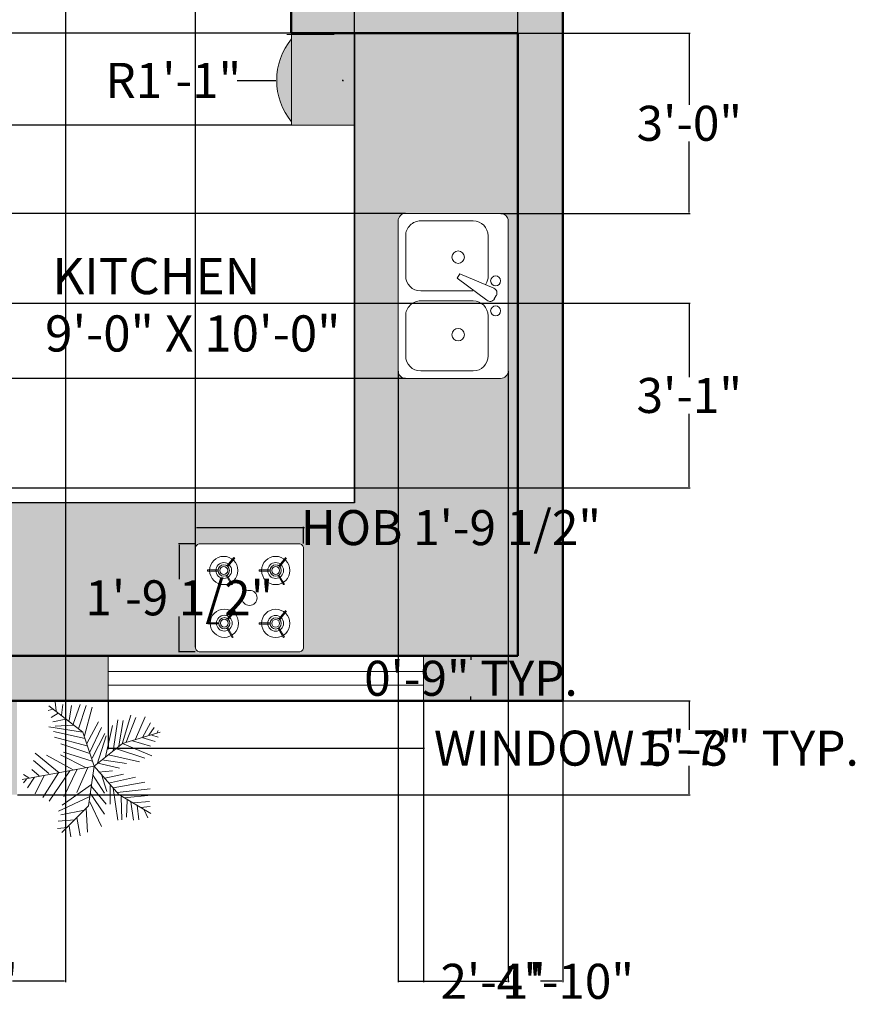
# Model space of a CAD drawing. Units: inches. Extents: x 2974 to 3443, y 2405 to 2963.
# Tile 6 of 13: x 3276 to 3443, y 2411 to 2607. Entities that reach past the tile are written whole.
import ezdxf

# ---------------------------------------------------------------- set-up
doc = ezdxf.new("R2010")
doc.units = ezdxf.units.IN
doc.header["$MEASUREMENT"] = 0
doc.layers.get('0').update_dxf_attribs({"color": 251})
for name, color, linetype, lineweight in [('A-ANNO-DIMS', 2, 'Continuous', 18), ('A-AREA-IDEN', 250, 'Continuous', 25), ('A-EQPM', 32, 'Continuous', 20), ('A-EQPM-PATT', 251, 'Continuous', 13), ('A-FLOR-CASE', 32, 'Continuous', 25), ('A-FLOR-CASE-PATT', 9, 'Continuous', 13), ('A-FLOR-FIXT', 8, 'Continuous', 20), ('A-WALL-PATT', 252, 'Continuous', 13), ('furniture', 32, 'Continuous', 18), ('greenary', 106, 'Continuous', 13), ('walls', 250, 'Continuous', 50), ('windows', 159, 'Continuous', 20)]:
    doc.layers.add(name, color=color, linetype=linetype, lineweight=lineweight)
doc.styles.add('ATT', font='TXT')
doc.styles.get("Standard").update_dxf_attribs({"font": 'arial.ttf'})
doc.dimstyles.get("Standard").update_dxf_attribs({"dimtxt": 7, "dimasz": 0.18, "dimexe": 0.18, "dimexo": 0.0625, "dimgap": 0.09, "dimtad": 0, "dimtih": 1, "dimtoh": 1, "dimzin": 0, "dimdsep": 46, "dimlunit": 3, "dimtxsty": 'Standard', "dimcen": 0.09, "dimadec": 0, "dimazin": 0, "dimtfac": 1, "dimtofl": 0, "dimtmove": 0, "dimatfit": 3, "dimfxl": 1, "dimtolj": 1, "dimtzin": 0, "dimarcsym": 0})

# ---------------------------------------------------------------- blocks, each defined once
blk = doc.blocks.new('15PSNK10')
at = {"color": 0, "linetype": 'ByBlock'}
for p, q in [((20.5, 16.5), (1.5, 16.5)), ((0, 15), (0, -15)), ((7, 15), (17.5, 15)), ((22, -15), (22, 15)), ((4, 4), (4, 12)), ((20.5, 12), (20.5, 4)), ((2.37, -0.1), (2.77, 0.6)), ((10.18, -3.57), (4.27, 0.87)), ((17.5, 1), (7, 1)), ((2.88, -1.54), (9.68, -4.43)), ((7.04, -1), (17.5, -1)), ((9.68, -4.43), (10.18, -3.57)), ((4, -12), (4, -4)), ((20.5, -4), (20.5, -12)), ((17.5, -15), (7, -15)), ((1.5, -16.5), (20.5, -16.5))]:
    blk.add_line(p, q, dxfattribs=at)
for centre, radius in [((10, 7.75), 1.25), ((2.5, 3), 1), ((2.5, -3), 1), ((10, -7.75), 1.25)]:
    blk.add_circle(centre, radius, dxfattribs=at)
for centre, radius, start, end in [((1.5, 15), 1.5, 90, 180), ((20.5, 15), 1.5, 0, 90), ((7, 12), 3, 90, 180), ((17.5, 12), 3, 0, 90), ((7, 4), 3, 180, 270), ((17.5, 4), 3, 270, 0), ((3.63, 0.1), 1, 50.5377, 150), ((3.23, -0.6), 1, 150, 249.4623), ((17.5, -4), 3, 0, 90), ((7, -4), 3, 146.607, 180), ((7, -12), 3, 180, 270), ((17.5, -12), 3, 270, 0), ((1.5, -15), 1.5, 180, 270), ((20.5, -15), 1.5, 270, 0)]:
    blk.add_arc(centre, radius, start, end, dxfattribs=at)
at = {"color": 0, "linetype": 'ByBlock', "style": 'ATT'}
for tag, p, flags in [('ITEM', (0, -26), 3), ('ROOM_NUMBER', (0, -35), 1)]:
    blk.add_attdef(tag, p, '', height=6, dxfattribs=dict(at, flags=flags))
blk = doc.blocks.new('4bstove')
at = {"layer": 'furniture'}
for p, q in [((1452.73, 1446.21), (1452.73, 1448.61)), ((1452.98, 1446.22), (1452.98, 1448.61)), ((1464.44, 1446.34), (1464.44, 1448.73)), ((1464.69, 1446.34), (1464.69, 1448.73)), ((1451.74, 1444.45), (1449.67, 1443.25)), ((1451.87, 1444.23), (1449.79, 1443.04)), ((1453.75, 1444.08), (1455.58, 1442.54)), ((1453.91, 1444.27), (1455.74, 1442.73)), ((1463.45, 1444.58), (1461.38, 1443.38)), ((1463.57, 1444.36), (1461.5, 1443.17)), ((1465.46, 1444.21), (1467.29, 1442.67)), ((1465.62, 1444.4), (1467.45, 1442.86)), ((1452.69, 1434.81), (1452.69, 1437.2)), ((1452.94, 1434.81), (1452.94, 1437.2)), ((1464.44, 1434.81), (1464.44, 1437.2)), ((1464.69, 1434.81), (1464.69, 1437.2)), ((1451.7, 1433.04), (1449.63, 1431.85)), ((1451.82, 1432.83), (1449.75, 1431.63)), ((1453.87, 1432.86), (1455.7, 1431.33)), ((1463.45, 1433.04), (1461.38, 1431.85)), ((1463.57, 1432.83), (1461.5, 1431.63)), ((1465.62, 1432.86), (1467.45, 1431.33)), ((1453.71, 1432.67), (1455.54, 1431.13)), ((1465.46, 1432.67), (1467.29, 1431.13))]:
    blk.add_line(p, q, dxfattribs=at)
for points in [[(1447.5, 1427.38), (1469.5, 1427.38, 0.414214), (1470.5, 1428.38), (1470.5, 1450.38, 0.414214), (1469.5, 1451.38), (1447.5, 1451.38, 0.414214), (1446.5, 1450.38), (1446.5, 1428.38, 0.414214)], [(1465.46, 1445.1, 1), (1463.71, 1445.1, 1)], [(1453.75, 1444.97, 1), (1452, 1444.97, 1)], [(1453.71, 1433.56, 1), (1451.96, 1433.56, 1)], [(1465.46, 1433.56, 1), (1463.71, 1433.56, 1)]]:
    blk.add_lwpolyline(points, format="xyb", close=True, dxfattribs=at)
for points in [[(1454.12, 1444.97, 1), (1451.62, 1444.97, 1), (1454.12, 1444.97, 1)], [(1465.83, 1445.1, 1), (1463.33, 1445.1, 1), (1465.83, 1445.1, 1)], [(1454.08, 1433.56, 1), (1451.58, 1433.56, 1), (1454.08, 1433.56, 1)], [(1465.83, 1433.56, 1), (1463.33, 1433.56, 1), (1465.83, 1433.56, 1)]]:
    blk.add_lwpolyline(points, format="xyb", dxfattribs=at)
for centre, radius in [((1452.87, 1444.97), 3.14), ((1464.58, 1445.1), 3.14), ((1452.87, 1444.97), 1.75), ((1464.58, 1445.1), 1.75), ((1458.5, 1439.38), 1.67), ((1452.83, 1433.56), 3.14), ((1452.83, 1433.56), 1.75), ((1464.58, 1433.56), 3.14), ((1464.58, 1433.56), 1.75)]:
    blk.add_circle(centre, radius, dxfattribs=at)
for centre, start, end in [((1452.87, 1444.97), 88.2645, 92.2039), ((1464.58, 1445.1), 88.2645, 92.2039), ((1452.87, 1444.97), 208.188, 212.1274), ((1452.87, 1444.97), 318.1018, 322.0412), ((1464.58, 1445.1), 208.188, 212.1274), ((1464.58, 1445.1), 318.1018, 322.0412), ((1452.83, 1433.56), 88.2645, 92.2039), ((1464.58, 1433.56), 88.2645, 92.2039)]:
    blk.add_arc(centre, 3.64, start, end, dxfattribs=at)
blk = doc.blocks.new('stove')
at = {"layer": 'furniture', "xscale": 0.9, "yscale": 0.9, "zscale": 0.9, "rotation": 89.99999999999999}
blk.add_blockref('4bstove', (1295.44, -1312.65), dxfattribs=at)
blk = doc.blocks.new('*U13')
for p, q in [((-10.186, 53.64), (-13.084, 55.962)), ((0, 0), (-10.5, 57)), ((-9.099, 51.782), (-6.563, 55.962)), ((-8.737, 47.138), (-17.069, 52.711)), ((-7.65, 43.423), (-2.578, 49.46)), ((-5.839, 35.992), (4.667, 48.067)), ((-5.114, 28.097), (-24.676, 40.636)), ((-7.288, 39.707), (-21.778, 46.673)), ((-5.114, 27.632), (10.463, 46.673)), ((-3.665, 19.273), (-27.574, 35.527)), ((-2.941, 16.486), (8.652, 37.85)), ((16.259, 5.805), (23.142, 31.348)), ((22.055, 7.198), (27.489, 32.277)), ((27, 9), (48, 36)), ((27.127, 9.056), (31.112, 35.992)), ((35.096, 32.741), (37.27, 22.524)), ((38.719, 34.134), (41.979, 28.561)), ((44.153, 36.456), (45.239, 32.741)), ((-31.5, 4.5), (-52.5, 25.5)), ((-48.585, 21.131), (-49.309, 29.026)), ((-43.513, 28.561), (-42.427, 15.558)), ((-38.442, 26.239), (-34.819, 7.663)), ((-35.544, 28.097), (-24.314, 3.947)), ((-14.533, 2.09), (-30.834, 25.31)), ((-24.314, 23.917), (-2.941, 13.7)), ((-1.129, 6.734), (9.014, 26.704)), ((3.942, 1.625), (11.187, 24.381)), ((10.101, 3.483), (17.708, 26.239)), ((31.836, 30.883), (32.561, 16.486)), ((40.53, 25.775), (48.862, 24.846)), ((43.791, 29.954), (51.036, 30.883)), ((-47.498, 19.737), (-55.83, 18.344)), ((33.285, 16.486), (48.862, 10.913)), ((36.183, 19.737), (48.137, 17.88)), ((-40.615, 13.7), (-55.105, 10.913)), ((-20.691, 13.7), (-1.129, 4.876)), ((0, 0), (27, 9)), ((29.662, 12.307), (48.137, 6.269)), ((-33.37, 6.269), (-52.207, 5.34)), ((-28.299, 3.483), (-47.86, -5.805)), ((-21.416, 3.018), (-38.079, -8.128)), ((0, 0), (-31.5, 4.5)), ((-15.982, 2.09), (-30.11, -9.521)), ((0, 0), (-22.5, -19.5)), ((-6.563, 1.161), (-21.416, -8.128)), ((0, 0), (18, -22.5)), ((6.478, 1.625), (26.04, -8.592)), ((11.187, 3.483), (30.749, -5.805)), ((18.07, 5.805), (35.096, -3.483)), ((24.229, 7.663), (46.688, 1.625)), ((-6.563, -5.805), (-19.967, -9.985)), ((-4.752, -3.483), (-3.665, -14.629)), ((2.493, -3.019), (-1.491, -20.202)), ((1.769, -2.555), (24.229, -9.521)), ((5.029, -6.27), (2.131, -25.775)), ((-17.431, -15.094), (-42.789, -18.809)), ((-15.257, -12.772), (-30.11, -12.772)), ((-17.069, -15.094), (-12.721, -40.172)), ((-13.446, -11.378), (-8.737, -32.741)), ((-9.461, -8.592), (-6.201, -23.453)), ((9.014, -11.378), (3.58, -35.992)), ((7.565, -9.056), (32.198, -14.629)), ((12.274, -15.094), (36.907, -18.809)), ((-24.314, -21.596), (-42.427, -22.06)), ((-22.5, -19.5), (-37.5, -45)), ((-20.691, -18.345), (-17.793, -44.352)), ((14.085, -16.951), (6.478, -40.172)), ((18.07, -22.524), (8.289, -45.745)), ((16.259, -19.738), (36.183, -22.989)), ((18, -22.5), (27, -52.5)), ((18.433, -22.524), (40.53, -29.026)), ((-28.299, -29.026), (-42.789, -31.348)), ((-26.849, -26.24), (-40.253, -25.775)), ((-29.023, -30.884), (-27.936, -43.887)), ((-25.038, -23.918), (-22.865, -45.281)), ((20.244, -30.419), (15.897, -44.816)), ((19.157, -25.311), (38.719, -33.206)), ((-30.834, -34.135), (-42.427, -35.528)), ((-32.646, -36.921), (-31.921, -44.352)), ((22.78, -37.85), (19.519, -48.532)), ((21.331, -32.741), (39.081, -40.636)), ((22.78, -38.314), (34.372, -44.816)), ((-34.457, -39.708), (-40.978, -42.494)), ((24.591, -45.745), (23.142, -50.854)), ((24.591, -43.423), (30.749, -47.603)), ((26.764, -49.925), (28.213, -50.854))]:
    blk.add_line(p, q)
blk = doc.blocks.new('WIN-63IN')
for p, q in [((0, 0), (0, -9)), ((63.13, 0), (0, 0)), ((0, 0), (0, -3.12)), ((63.13, -9), (63.13, 0)), ((0, -3.12), (63.13, -3.12)), ((63.13, -3.12), (63.13, -5.89)), ((63.13, -5.89), (0, -5.89)), ((0, -9), (63.13, -9))]:
    blk.add_line(p, q)
blk = doc.blocks.new('*D39')
at = {"layer": 'A-ANNO-DIMS', "color": 0, "lineweight": -2, "transparency": 16777216}
for p, q in [((3293.36, 2471.13), (3293.36, 2461.54)), ((3356.49, 2471.13), (3356.49, 2461.54)), ((3293.54, 2461.72), (3356.31, 2461.72)), ((3356.49, 2461.72), (3356.67, 2461.72))]:
    blk.add_line(p, q, dxfattribs=at)
at = {"layer": 'A-ANNO-DIMS', "color": 0, "transparency": 16777216}
for points in [[(3293.54, 2461.75), (3293.54, 2461.69), (3293.36, 2461.72)], [(3356.31, 2461.75), (3356.31, 2461.69), (3356.49, 2461.72)]]:
    blk.add_solid(points, dxfattribs=at)
at = {"layer": 'Defpoints', "color": 0, "transparency": 16777216}
for p in [(3293.36, 2471.19), (3356.49, 2471.19), (3356.49, 2461.72)]:
    blk.add_point(p, dxfattribs=at)
at = {"layer": 'A-ANNO-DIMS', "color": 0, "transparency": 16777216, "insert": (3401.05, 2461.72), "char_height": 7, "attachment_point": 5}
blk.add_mtext('\\A1;WINDOW 5\'-3" TYP.', dxfattribs=at)
blk = doc.blocks.new('*D40')
at = {"layer": 'A-ANNO-DIMS', "color": 0, "lineweight": -2, "transparency": 16777216}
for p, q in [((3356.55, 2480.19), (3366.14, 2480.19)), ((3365.96, 2480.01), (3365.96, 2479.35)), ((3356.55, 2471.19), (3366.14, 2471.19)), ((3365.96, 2471.37), (3365.96, 2472.02))]:
    blk.add_line(p, q, dxfattribs=at)
at = {"layer": 'A-ANNO-DIMS', "color": 0, "transparency": 16777216}
for points in [[(3365.93, 2480.01), (3365.99, 2480.01), (3365.96, 2480.19)], [(3365.93, 2471.37), (3365.99, 2471.37), (3365.96, 2471.19)]]:
    blk.add_solid(points, dxfattribs=at)
at = {"layer": 'Defpoints', "color": 0, "transparency": 16777216}
for p in [(3356.49, 2480.19), (3365.96, 2480.19), (3356.49, 2471.19)]:
    blk.add_point(p, dxfattribs=at)
at = {"layer": 'A-ANNO-DIMS', "color": 0, "transparency": 16777216, "insert": (3365.96, 2475.69), "char_height": 7, "attachment_point": 5}
blk.add_mtext('\\A1;0\'-9" TYP.', dxfattribs=at)
blk = doc.blocks.new('*D43')
at = {"layer": 'A-ANNO-DIMS', "color": 0, "lineweight": -2, "transparency": 16777216}
for p, q in [((3310.86, 2502.63), (3310.86, 2505.99)), ((3311.04, 2505.81), (3332.28, 2505.81)), ((3332.46, 2502.63), (3332.46, 2505.99)), ((3332.46, 2505.81), (3332.64, 2505.81))]:
    blk.add_line(p, q, dxfattribs=at)
at = {"layer": 'A-ANNO-DIMS', "color": 0, "transparency": 16777216}
for points in [[(3311.04, 2505.84), (3311.04, 2505.78), (3310.86, 2505.81)], [(3332.28, 2505.84), (3332.28, 2505.78), (3332.46, 2505.81)]]:
    blk.add_solid(points, dxfattribs=at)
at = {"layer": 'Defpoints', "color": 0, "transparency": 16777216}
for p in [(3332.46, 2505.81), (3310.86, 2502.57), (3332.46, 2502.57)]:
    blk.add_point(p, dxfattribs=at)
at = {"layer": 'A-ANNO-DIMS', "color": 0, "transparency": 16777216, "insert": (3361.96, 2505.81), "char_height": 7, "attachment_point": 5}
blk.add_mtext('\\A1;HOB 1\'-9 1/2"', dxfattribs=at)
blk = doc.blocks.new('*D44')
at = {"layer": 'A-ANNO-DIMS', "color": 0, "lineweight": -2, "transparency": 16777216}
for p, q in [((3310.8, 2502.57), (3307.44, 2502.57)), ((3307.62, 2502.39), (3307.62, 2495.48)), ((3307.62, 2481.15), (3307.62, 2488.06)), ((3310.8, 2480.97), (3307.44, 2480.97))]:
    blk.add_line(p, q, dxfattribs=at)
at = {"layer": 'A-ANNO-DIMS', "color": 0, "transparency": 16777216}
for points in [[(3307.59, 2502.39), (3307.65, 2502.39), (3307.62, 2502.57)], [(3307.59, 2481.15), (3307.65, 2481.15), (3307.62, 2480.97)]]:
    blk.add_solid(points, dxfattribs=at)
at = {"layer": 'Defpoints', "color": 0, "transparency": 16777216}
for p in [(3307.62, 2502.57), (3310.86, 2502.57), (3310.86, 2480.97)]:
    blk.add_point(p, dxfattribs=at)
at = {"layer": 'A-ANNO-DIMS', "color": 0, "transparency": 16777216, "insert": (3307.62, 2491.77), "char_height": 7, "attachment_point": 5}
blk.add_mtext('\\A1;1\'-9 1/2"', dxfattribs=at)
blk = doc.blocks.new('*D57')
at = {"layer": 'A-ANNO-DIMS', "color": 0, "lineweight": -2, "transparency": 16777216}
for p, q in [((3356.49, 2471.13), (3356.49, 2414.92)), ((3384.33, 2471.13), (3384.33, 2414.92)), ((3356.67, 2415.1), (3360.95, 2415.1)), ((3384.15, 2415.1), (3379.86, 2415.1))]:
    blk.add_line(p, q, dxfattribs=at)
at = {"layer": 'A-ANNO-DIMS', "color": 0, "transparency": 16777216}
for points in [[(3356.67, 2415.13), (3356.67, 2415.07), (3356.49, 2415.1)], [(3384.15, 2415.13), (3384.15, 2415.07), (3384.33, 2415.1)]]:
    blk.add_solid(points, dxfattribs=at)
at = {"layer": 'Defpoints', "color": 0, "transparency": 16777216}
for p in [(3356.49, 2471.19), (3384.33, 2471.19), (3384.33, 2415.1)]:
    blk.add_point(p, dxfattribs=at)
at = {"layer": 'A-ANNO-DIMS', "color": 0, "transparency": 16777216, "insert": (3370.41, 2415.1), "char_height": 7, "attachment_point": 5}
blk.add_mtext('\\A1;2\'-4"', dxfattribs=at)
blk = doc.blocks.new('*D60')
at = {"layer": 'A-ANNO-DIMS', "color": 0, "lineweight": -2, "transparency": 16777216}
for p, q in [((3275.25, 2471.19), (3409.82, 2471.19)), ((3409.64, 2471.01), (3409.64, 2465.41)), ((3409.64, 2452.59), (3409.64, 2458.2)), ((3275.25, 2452.41), (3409.82, 2452.41))]:
    blk.add_line(p, q, dxfattribs=at)
at = {"layer": 'A-ANNO-DIMS', "color": 0, "transparency": 16777216}
for points in [[(3409.61, 2471.01), (3409.67, 2471.01), (3409.64, 2471.19)], [(3409.61, 2452.59), (3409.67, 2452.59), (3409.64, 2452.41)]]:
    blk.add_solid(points, dxfattribs=at)
at = {"layer": 'Defpoints', "color": 0, "transparency": 16777216}
for p in [(3275.19, 2471.19), (3409.64, 2471.19), (3275.19, 2452.41)]:
    blk.add_point(p, dxfattribs=at)
at = {"layer": 'A-ANNO-DIMS', "color": 0, "transparency": 16777216, "insert": (3409.64, 2461.8), "char_height": 7, "attachment_point": 5}
blk.add_mtext('\\A1;1\'-7"', dxfattribs=at)
blk = doc.blocks.new('*D63')
at = {"layer": 'A-ANNO-DIMS', "color": 0, "lineweight": -2, "transparency": 16777216}
for p, q in [((3244.83, 2751.13), (3244.83, 2414.92)), ((3284.83, 2751.13), (3284.83, 2414.92)), ((3245.01, 2415.1), (3255.43, 2415.1)), ((3284.65, 2415.1), (3274.22, 2415.1))]:
    blk.add_line(p, q, dxfattribs=at)
at = {"layer": 'A-ANNO-DIMS', "color": 0, "transparency": 16777216}
for points in [[(3245.01, 2415.13), (3245.01, 2415.07), (3244.83, 2415.1)], [(3284.65, 2415.13), (3284.65, 2415.07), (3284.83, 2415.1)]]:
    blk.add_solid(points, dxfattribs=at)
at = {"layer": 'Defpoints', "color": 0, "transparency": 16777216}
for p in [(3244.83, 2751.19), (3284.83, 2751.19), (3284.83, 2415.1)]:
    blk.add_point(p, dxfattribs=at)
at = {"layer": 'A-ANNO-DIMS', "color": 0, "transparency": 16777216, "insert": (3264.83, 2415.1), "char_height": 7, "attachment_point": 5}
blk.add_mtext('\\A1;3\'-4"', dxfattribs=at)
blk = doc.blocks.new('*D67')
at = {"layer": 'A-ANNO-DIMS', "color": 0, "lineweight": -2, "transparency": 16777216}
for p, q in [((3170.07, 2550.69), (3409.82, 2550.69)), ((3409.64, 2550.51), (3409.64, 2535.9)), ((3409.64, 2513.97), (3409.64, 2528.57)), ((3170.07, 2513.79), (3409.82, 2513.79))]:
    blk.add_line(p, q, dxfattribs=at)
at = {"layer": 'A-ANNO-DIMS', "color": 0, "transparency": 16777216}
for points in [[(3409.61, 2550.51), (3409.67, 2550.51), (3409.64, 2550.69)], [(3409.61, 2513.97), (3409.67, 2513.97), (3409.64, 2513.79)]]:
    blk.add_solid(points, dxfattribs=at)
at = {"layer": 'Defpoints', "color": 0, "transparency": 16777216}
for p in [(3170, 2550.69), (3409.64, 2550.69), (3170, 2513.79)]:
    blk.add_point(p, dxfattribs=at)
at = {"layer": 'A-ANNO-DIMS', "color": 0, "transparency": 16777216, "insert": (3409.64, 2532.24), "char_height": 7, "attachment_point": 5}
blk.add_mtext('\\A1;3\'-1"', dxfattribs=at)
blk = doc.blocks.new('*D72')
at = {"layer": 'A-ANNO-DIMS', "color": 0, "lineweight": -2, "transparency": 16777216}
for p, q in [((3342.69, 2510.82), (3342.69, 2952.68)), ((3342.87, 2952.5), (3375.15, 2952.5)), ((3375.33, 2480.25), (3375.33, 2952.68)), ((3375.33, 2952.5), (3375.51, 2952.5))]:
    blk.add_line(p, q, dxfattribs=at)
at = {"layer": 'A-ANNO-DIMS', "color": 0, "transparency": 16777216}
for points in [[(3342.87, 2952.53), (3342.87, 2952.47), (3342.69, 2952.5)], [(3375.15, 2952.53), (3375.15, 2952.47), (3375.33, 2952.5)]]:
    blk.add_solid(points, dxfattribs=at)
at = {"layer": 'Defpoints', "color": 0, "transparency": 16777216}
for p in [(3375.33, 2952.5), (3342.69, 2510.76), (3375.33, 2480.19)]:
    blk.add_point(p, dxfattribs=at)
at = {"layer": 'A-ANNO-DIMS', "color": 0, "transparency": 16777216, "insert": (3393.11, 2952.5), "char_height": 7, "attachment_point": 5}
blk.add_mtext('\\A1;2\'-8 1/2"', dxfattribs=at)
blk = doc.blocks.new('*D73')
at = {"layer": 'A-ANNO-DIMS', "color": 0, "lineweight": -2, "transparency": 16777216}
for p, q in [((3329.94, 2604.69), (2992.84, 2604.69)), ((2993.02, 2604.51), (2993.02, 2599.19)), ((2993.02, 2586.45), (2993.02, 2591.77)), ((3330, 2586.27), (2992.84, 2586.27))]:
    blk.add_line(p, q, dxfattribs=at)
at = {"layer": 'A-ANNO-DIMS', "color": 0, "transparency": 16777216}
for points in [[(2992.99, 2604.51), (2993.05, 2604.51), (2993.02, 2604.69)], [(2992.99, 2586.45), (2993.05, 2586.45), (2993.02, 2586.27)]]:
    blk.add_solid(points, dxfattribs=at)
at = {"layer": 'Defpoints', "color": 0, "transparency": 16777216}
for p in [(2993.02, 2604.69), (3330, 2604.69), (3330.06, 2586.27)]:
    blk.add_point(p, dxfattribs=at)
at = {"layer": 'A-ANNO-DIMS', "color": 0, "transparency": 16777216, "insert": (2993.02, 2595.48), "char_height": 7, "attachment_point": 5}
blk.add_mtext('\\A1;1\'-6 1/2"', dxfattribs=at)
blk = doc.blocks.new('*D75')
at = {"layer": 'A-ANNO-DIMS', "color": 0, "lineweight": -2, "transparency": 16777216}
for p, q in [((3351.4, 2537.08), (3351.4, 2414.92)), ((3373.4, 2537.08), (3373.4, 2414.92)), ((3351.58, 2415.1), (3373.22, 2415.1)), ((3373.4, 2415.1), (3373.58, 2415.1))]:
    blk.add_line(p, q, dxfattribs=at)
at = {"layer": 'A-ANNO-DIMS', "color": 0, "transparency": 16777216}
for points in [[(3351.58, 2415.13), (3351.58, 2415.07), (3351.4, 2415.1)], [(3373.22, 2415.13), (3373.22, 2415.07), (3373.4, 2415.1)]]:
    blk.add_solid(points, dxfattribs=at)
at = {"layer": 'Defpoints', "color": 0, "transparency": 16777216}
for p in [(3351.4, 2537.14), (3373.4, 2537.14), (3373.4, 2415.1)]:
    blk.add_point(p, dxfattribs=at)
at = {"layer": 'A-ANNO-DIMS', "color": 0, "transparency": 16777216, "insert": (3385.37, 2415.1), "char_height": 7, "attachment_point": 5}
blk.add_mtext('\\A1;1\'-10"', dxfattribs=at)
blk = doc.blocks.new('*D76')
at = {"layer": 'A-ANNO-DIMS', "color": 0, "lineweight": -2, "transparency": 16777216}
for p, q in [((3352.84, 2568.64), (2992.84, 2568.64)), ((2993.02, 2568.46), (2993.02, 2555.8)), ((2993.02, 2535.82), (2993.02, 2548.48)), ((3352.84, 2535.64), (2992.84, 2535.64))]:
    blk.add_line(p, q, dxfattribs=at)
at = {"layer": 'A-ANNO-DIMS', "color": 0, "transparency": 16777216}
for points in [[(2992.99, 2568.46), (2993.05, 2568.46), (2993.02, 2568.64)], [(2992.99, 2535.82), (2993.05, 2535.82), (2993.02, 2535.64)]]:
    blk.add_solid(points, dxfattribs=at)
at = {"layer": 'Defpoints', "color": 0, "transparency": 16777216}
for p in [(2993.02, 2568.64), (3352.9, 2568.64), (3352.9, 2535.64)]:
    blk.add_point(p, dxfattribs=at)
at = {"layer": 'A-ANNO-DIMS', "color": 0, "transparency": 16777216, "insert": (2993.02, 2552.14), "char_height": 7, "attachment_point": 5}
blk.add_mtext('\\A1;2\'-9"', dxfattribs=at)
blk = doc.blocks.new('*D77')
at = {"layer": 'A-ANNO-DIMS', "color": 0, "lineweight": -2, "transparency": 16777216}
for p, q in [((3375.39, 2604.69), (3409.82, 2604.69)), ((3409.64, 2604.51), (3409.64, 2590.33)), ((3409.64, 2568.82), (3409.64, 2583)), ((3371.97, 2568.64), (3409.82, 2568.64))]:
    blk.add_line(p, q, dxfattribs=at)
at = {"layer": 'A-ANNO-DIMS', "color": 0, "transparency": 16777216}
for points in [[(3409.61, 2604.51), (3409.67, 2604.51), (3409.64, 2604.69)], [(3409.61, 2568.82), (3409.67, 2568.82), (3409.64, 2568.64)]]:
    blk.add_solid(points, dxfattribs=at)
at = {"layer": 'Defpoints', "color": 0, "transparency": 16777216}
for p in [(3375.33, 2604.69), (3371.9, 2568.64), (3409.64, 2568.64)]:
    blk.add_point(p, dxfattribs=at)
at = {"layer": 'A-ANNO-DIMS', "color": 0, "transparency": 16777216, "insert": (3409.64, 2586.66), "char_height": 7, "attachment_point": 5}
blk.add_mtext('\\A1;3\'-0"', dxfattribs=at)
blk = doc.blocks.new('*D78')
at = {"layer": 'A-ANNO-DIMS', "color": 0, "lineweight": -2, "transparency": 16777216}
for p, q in [((3267.33, 2480.25), (3267.33, 2952.68)), ((3267.51, 2952.5), (3271.55, 2952.5)), ((3310.68, 2952.5), (3306.64, 2952.5)), ((3310.86, 2481.93), (3310.86, 2952.68))]:
    blk.add_line(p, q, dxfattribs=at)
at = {"layer": 'A-ANNO-DIMS', "color": 0, "transparency": 16777216}
for points in [[(3267.51, 2952.53), (3267.51, 2952.47), (3267.33, 2952.5)], [(3310.68, 2952.53), (3310.68, 2952.47), (3310.86, 2952.5)]]:
    blk.add_solid(points, dxfattribs=at)
at = {"layer": 'Defpoints', "color": 0, "transparency": 16777216}
for p in [(3310.86, 2952.5), (3310.86, 2481.87), (3267.33, 2480.19)]:
    blk.add_point(p, dxfattribs=at)
at = {"layer": 'A-ANNO-DIMS', "color": 0, "transparency": 16777216, "insert": (3289.09, 2952.5), "char_height": 7, "attachment_point": 5}
blk.add_mtext('\\A1;3\'-7 1/2"', dxfattribs=at)
blk = doc.blocks.new('*D79')
at = {"layer": 'A-ANNO-DIMS', "color": 0, "lineweight": -2, "transparency": 16777216}
for p, q in [((3319.17, 2595.24), (3326.93, 2595.24)), ((3340.26, 2595.24), (3340.44, 2595.24)), ((3340.35, 2595.15), (3340.35, 2595.33))]:
    blk.add_line(p, q, dxfattribs=at)
at = {"layer": 'A-ANNO-DIMS', "color": 0, "transparency": 16777216}
blk.add_solid([(3326.93, 2595.27), (3326.93, 2595.21), (3327.11, 2595.24)], dxfattribs=at)
at = {"layer": 'Defpoints', "color": 0, "transparency": 16777216}
for p in [(3327.11, 2595.24), (3340.35, 2595.24)]:
    blk.add_point(p, dxfattribs=at)
at = {"layer": 'A-ANNO-DIMS', "color": 0, "transparency": 16777216, "insert": (3306.42, 2595.24), "char_height": 7, "attachment_point": 5}
blk.add_mtext('\\A1;R1\'-1"', dxfattribs=at)

msp = doc.modelspace()

# ---------------------------------------------------------------- hatches: boundary and pattern name
at = {"layer": 'A-EQPM-PATT'}
h = msp.add_hatch(color=256, dxfattribs=at)
h.dxf.hatch_style = 1
h.paths.add_polyline_path([(3342.691, 2604.438), (3330.059, 2604.438), (3330.059, 2586.273), (3342.691, 2586.273)])
h.paths.add_polyline_path([(3330.059, 2603.573, 0.3538958), (3330.059, 2586.914)])
at = {"layer": 'A-FLOR-CASE-PATT'}
h = msp.add_hatch(color=256, dxfattribs=at)
h.dxf.hatch_style = 1
h.paths.add_polyline_path([(3375.326, 2480.188), (3267.326, 2480.188), (3267.326, 2510.762), (3342.691, 2510.762), (3342.691, 2604.688), (3375.326, 2604.688)])
h.paths.add_polyline_path([(3332.464, 2481.869, -0.4142136), (3331.564, 2480.969), (3311.764, 2480.969, -0.4142136), (3310.864, 2481.869), (3310.864, 2501.669, -0.4142136), (3311.764, 2502.569), (3331.564, 2502.569, -0.4142136), (3332.464, 2501.669)], flags=16)
h.paths.add_polyline_path([(3324.078, 2497.114), (3323.628, 2497.114, -0.0171907), (3323.627, 2497.339), (3324.077, 2497.339, -0.9825922), (3329.722, 2497.24, -0.9779445)], flags=0)
h.paths.add_polyline_path([(3328.474, 2497.24, -1), (3325.324, 2497.24, -1)], flags=0)
h.paths.add_polyline_path([(3326.899, 2496.115, -1), (3326.899, 2498.365, -1)], flags=0)
h.paths.add_polyline_path([(3326.899, 2496.453, -1), (3326.899, 2498.028, -1)], flags=0)
h.paths.add_polyline_path([(3329.722, 2486.666, -0.9779445), (3324.078, 2486.54), (3323.628, 2486.54, -0.0171907), (3323.627, 2486.765), (3324.077, 2486.765, -0.9825922)], flags=0)
h.paths.add_polyline_path([(3328.474, 2486.666, -1), (3325.324, 2486.666, -1)], flags=0)
h.paths.add_polyline_path([(3326.899, 2485.541, -1), (3326.899, 2487.791, -1)], flags=0)
h.paths.add_polyline_path([(3326.899, 2485.878, -1), (3326.899, 2487.453, -1)], flags=0)
h.paths.add_polyline_path([(3323.167, 2491.769, -1), (3320.16, 2491.769, -1)], flags=0)
h.paths.add_polyline_path([(3318.032, 2494.858), (3318.257, 2494.468, -0.0171907), (3318.063, 2494.355), (3317.838, 2494.745, -0.5505708), (3313.696, 2497.114), (3313.246, 2497.114, -0.0171907), (3313.245, 2497.339), (3313.695, 2497.339, -0.6105283), (3318.24, 2499.476), (3318.53, 2499.821, -0.0171906), (3318.702, 2499.677), (3318.413, 2499.332, -0.2116406), (3319.34, 2497.24, -0.2564461)], flags=0)
h.paths.add_polyline_path([(3314.942, 2497.24, -1), (3318.092, 2497.24, -1)], flags=0)
h.paths.add_polyline_path([(3316.517, 2496.115, -1), (3316.517, 2498.365, -1)], flags=0)
h.paths.add_polyline_path([(3318.817, 2489.141), (3318.528, 2488.796, -0.2116406), (3319.454, 2486.704, -0.2564461), (3318.147, 2484.322), (3318.372, 2483.932, -0.0171907), (3318.177, 2483.819), (3317.952, 2484.209, -0.5505708), (3313.811, 2486.578), (3313.361, 2486.578, -0.0171907), (3313.36, 2486.803), (3313.81, 2486.803, -0.6105283), (3318.355, 2488.94), (3318.645, 2489.285, -0.0171906)], flags=0)
h.paths.add_polyline_path([(3316.517, 2496.453, -1), (3316.517, 2498.028, -1)], flags=0)
h.paths.add_polyline_path([(3318.206, 2486.704, -1), (3315.056, 2486.704, -1)], flags=0)
h.paths.add_polyline_path([(3316.631, 2485.579, -1), (3316.631, 2487.829, -1)], flags=0)
h.paths.add_polyline_path([(3316.631, 2485.917, -1), (3316.631, 2487.492, -1)], flags=0)
h.paths.add_polyline_path([(3351.404, 2537.14), (3351.404, 2567.14, -0.4142136), (3352.904, 2568.64), (3371.904, 2568.64, -0.4142136), (3373.404, 2567.14), (3373.404, 2537.14, -0.4142136), (3371.904, 2535.64), (3352.904, 2535.64, -0.4142136)], flags=16)
h.paths.add_polyline_path([(3352.904, 2540.14), (3352.904, 2548.14, -0.4142136), (3355.904, 2551.14), (3366.404, 2551.14, -0.4142136), (3369.404, 2548.14), (3369.404, 2540.14, -0.4142136), (3366.404, 2537.14), (3355.904, 2537.14, -0.4142136)], flags=0)
h.paths.add_polyline_path([(3362.154, 2544.39, -1), (3364.654, 2544.39, -1)], flags=0)
h.paths.add_polyline_path([(3369.904, 2549.14, -1), (3371.904, 2549.14, -1)], flags=0)
h.paths.add_polyline_path([(3370.523, 2553.675, -0.4631995), (3371.039, 2552.239), (3370.636, 2551.542, -0.4369422), (3369.205, 2551.215), (3363.226, 2555.707), (3363.726, 2556.573)], flags=0)
h.paths.add_polyline_path([(3369.904, 2555.14, -1), (3371.904, 2555.14, -1)], flags=0)
h.paths.add_polyline_path([(3362.154, 2559.89, -1), (3364.654, 2559.89, -1)], flags=0)
at = {"layer": 'A-WALL-PATT'}
h = msp.add_hatch(color=256, dxfattribs=at)
h.dxf.hatch_style = 1
h.paths.add_polyline_path([(3222.294, 2555.188), (3211.826, 2555.188), (3211.826, 2657.938), (3207.326, 2657.938), (3207.326, 2555.188), (3051.326, 2555.188), (3051.326, 2583.943), (3042.326, 2583.943), (3042.326, 2471.188), (3165.027, 2471.188), (3165.027, 2480.188), (3051.326, 2480.188), (3051.326, 2550.688), (3222.294, 2550.688)])
h.paths.add_polyline_path([(3188.326, 2700.207), (3183.826, 2700.207), (3183.826, 2691.688), (3051.326, 2691.688), (3051.326, 2740.572), (3042.326, 2740.572), (3042.326, 2651.235), (3045.517, 2651.235), (3051.326, 2651.235), (3051.326, 2687.188), (3188.326, 2687.188)])
h.paths.add_polyline_path([(3051.326, 2894.188), (3074.298, 2894.188), (3074.298, 2903.188), (3042.326, 2903.188), (3042.326, 2807.864), (3045.517, 2807.864), (3051.326, 2807.864), (3051.326, 2835.688), (3103.457, 2835.688), (3103.457, 2839.066, -0.0124729), (3103.485, 2840.188), (3051.326, 2840.188)])
h.paths.add_polyline_path([(3201.987, 2903.188), (3100.263, 2903.188), (3100.263, 2894.188), (3131.326, 2894.188), (3131.326, 2835.688), (3135.826, 2835.688), (3135.826, 2894.188), (3183.826, 2894.188), (3183.826, 2840.188), (3159.826, 2840.188), (3159.826, 2835.688), (3183.826, 2835.688), (3183.826, 2740.207), (3188.326, 2740.207), (3188.326, 2803.688), (3215.422, 2803.688), (3215.422, 2807.066, -0.0124729), (3215.45, 2808.188), (3188.326, 2808.188), (3188.326, 2894.188), (3201.987, 2894.188)])
h.paths.add_polyline_path([(3283.564, 2903.188), (3227.952, 2903.188), (3227.952, 2894.188), (3240.326, 2894.188), (3240.326, 2755.688), (3188.326, 2755.688), (3188.326, 2751.188), (3244.826, 2751.188), (3244.826, 2757.188), (3244.826, 2797.188), (3244.826, 2894.188), (3283.564, 2894.188)])
h.paths.add_polyline_path([(3384.326, 2903.188), (3346.694, 2903.188), (3346.694, 2894.188), (3375.326, 2894.188), (3375.326, 2755.688), (3284.826, 2755.688), (3284.826, 2751.188), (3375.326, 2751.188), (3375.326, 2710.653), (3378.517, 2710.653), (3384.326, 2710.653)])
h.paths.add_polyline_path([(3384.326, 2643.361), (3375.326, 2643.361), (3375.326, 2609.188), (3330.003, 2609.188), (3330.003, 2604.688), (3375.326, 2604.688), (3375.326, 2480.188), (3356.49, 2480.188), (3356.49, 2471.188), (3384.326, 2471.188)])
h.paths.add_polyline_path([(3267.326, 2609.188), (3262.826, 2609.188), (3262.826, 2555.188), (3257.429, 2555.188), (3257.429, 2550.688), (3262.826, 2550.688), (3262.826, 2471.188), (3293.36, 2471.188), (3293.36, 2480.188), (3267.326, 2480.188)])
h.paths.add_polyline_path([(3275.186, 2471.188), (3268.471, 2471.188), (3268.471, 2455.229), (3268.471, 2452.413), (3275.186, 2452.413)])
h.paths.add_polyline_path([(3156.684, 2471.188), (3149.969, 2471.188), (3149.969, 2452.413), (3156.684, 2452.413)])

# ---------------------------------------------------------------- linework, layer by layer
at = {"layer": 'A-EQPM'}
for p, q in [((3329.157, 2604.438), (3338.624, 2604.438)), ((3330.059, 2586.273), (3330.059, 2604.438)), ((3342.691, 2604.438), (3342.691, 2586.273)), ((3342.691, 2586.273), (3330.059, 2586.273))]:
    msp.add_line(p, q, dxfattribs=at)
msp.add_arc((3340.353, 2595.243), 13.242, 141.02269, 218.97731, dxfattribs=at)
at = {"layer": 'A-FLOR-CASE'}
for p, q in [((3342.691, 2604.438), (3342.691, 2510.762)), ((3342.691, 2510.762), (3267.326, 2510.762))]:
    msp.add_line(p, q, dxfattribs=at)
at = {"layer": 'walls'}
for p, q in [((3384.326, 2903.188), (3384.326, 2471.188)), ((3330.003, 2609.188), (3330.003, 2604.688)), ((3330.003, 2604.688), (3375.326, 2604.688)), ((3375.326, 2604.688), (3375.326, 2480.188)), ((3375.326, 2480.188), (3267.326, 2480.188)), ((3384.326, 2471.188), (3262.826, 2471.188))]:
    msp.add_line(p, q, dxfattribs=at)

# ---------------------------------------------------------------- block references
at = {"layer": 'A-EQPM'}
msp.add_blockref('stove', (3321.664, 2491.769), dxfattribs=at)
at = {"layer": 'A-FLOR-FIXT', "rotation": 180}
msp.add_blockref('15PSNK10', (3373.404, 2552.14), dxfattribs=at)
at = {"layer": 'greenary', "xscale": 0.2522732792106678, "yscale": 0.2522732792106678, "zscale": 0.2522732792106678, "rotation": 90}
msp.add_blockref('*U13', (3290.573, 2458.103), dxfattribs=at)
at = {"layer": 'windows'}
msp.add_blockref('WIN-63IN', (3293.36, 2480.188), dxfattribs=at)

# ---------------------------------------------------------------- texts
at = {"layer": 'A-AREA-IDEN'}
for s, height, p in [('KITCHEN', 7.2272, (3282.247, 2552.488)), ('9\'-0" X 10\'-0"', 7.22716, (3280.768, 2541.019))]:
    msp.add_text(s, height=height, dxfattribs=at).set_placement(p)

# ---------------------------------------------------------------- dimensions: what is measured, and where the dimension line sits
at = {"layer": 'A-ANNO-DIMS'}
for base, p1, p2, picture, middle in [((3310.864, 2952.498), (3267.326, 2480.188), (3310.864, 2481.869), '*D78', (3289.095, 2952.498)), ((3375.326, 2952.498), (3342.691, 2510.762), (3375.326, 2480.188), '*D72', (3393.115, 2952.498)), ((3284.826, 2415.097), (3244.826, 2751.188), (3284.826, 2751.188), '*D63', (3264.826, 2415.097)), ((3373.404, 2415.097), (3351.404, 2537.14), (3373.404, 2537.14), '*D75', (3385.367, 2415.097)), ((3384.326, 2415.097), (3356.49, 2471.188), (3384.326, 2471.188), '*D57', (3370.408, 2415.097))]:
    dim = msp.add_linear_dim(base=base, p1=p1, p2=p2, dimstyle='Standard', override={"dimdec": 1, "dimlfac": 1, "dimrnd": 0, "dimzin": 1, "dimdsep": 46, "dimlunit": 4, "dimfrac": 2}, dxfattribs=at)
    dim.commit()
    dim.dimension.update_dxf_attribs({"geometry": picture, "text_midpoint": middle})
for base, p1, p2, picture, middle in [((2993.016, 2604.688), (3330.059, 2586.273), (3330.003, 2604.688), '*D73', (2993.016, 2595.481)), ((3409.636, 2568.64), (3375.326, 2604.688), (3371.904, 2568.64), '*D77', (3409.636, 2586.664)), ((2993.016, 2568.64), (3352.904, 2535.64), (3352.904, 2568.64), '*D76', (2993.016, 2552.14)), ((3409.636, 2550.688), (3170.003, 2513.788), (3170.003, 2550.688), '*D67', (3409.636, 2532.238)), ((3307.624, 2502.569), (3310.864, 2480.969), (3310.864, 2502.569), '*D44', (3307.624, 2491.769)), ((3409.636, 2471.188), (3275.186, 2452.413), (3275.186, 2471.188), '*D60', (3409.636, 2461.801))]:
    dim = msp.add_linear_dim(base=base, p1=p1, p2=p2, angle=90, dimstyle='Standard', override={"dimdec": 1, "dimlfac": 1, "dimrnd": 0, "dimzin": 1, "dimdsep": 46, "dimlunit": 4, "dimfrac": 2}, dxfattribs=at)
    dim.commit()
    dim.dimension.update_dxf_attribs({"geometry": picture, "text_midpoint": middle})
dim = msp.add_radius_dim(center=(3340.353, 2595.243), mpoint=(3327.111, 2595.243), dimstyle='Standard', override={"dimdec": 1, "dimlfac": 1, "dimrnd": 0, "dimzin": 1, "dimdsep": 46, "dimlunit": 4, "dimfrac": 2}, dxfattribs=at)
dim.commit()
dim.dimension.update_dxf_attribs({"geometry": '*D79', "text_midpoint": (3319.166, 2595.243), "dimtype": 164})
for base, p1, p2, text, picture, middle in [((3332.464, 2505.809), (3310.864, 2502.569), (3332.464, 2502.569), 'HOB <>', '*D43', (3361.959, 2505.809)), ((3356.49, 2461.719), (3293.36, 2471.188), (3356.49, 2471.188), 'WINDOW <> TYP.', '*D39', (3401.05, 2461.719))]:
    dim = msp.add_linear_dim(base=base, p1=p1, p2=p2, text=text, dimstyle='Standard', override={"dimdec": 1, "dimlfac": 1, "dimrnd": 0, "dimzin": 1, "dimdsep": 46, "dimlunit": 4, "dimfrac": 2}, dxfattribs=at)
    dim.commit()
    dim.dimension.update_dxf_attribs({"geometry": picture, "text_midpoint": middle})
dim = msp.add_linear_dim(base=(3365.96, 2480.188), p1=(3356.49, 2471.188), p2=(3356.49, 2480.188), angle=90, text='<> TYP.', dimstyle='Standard', override={"dimdec": 1, "dimlfac": 1, "dimrnd": 0, "dimzin": 1, "dimdsep": 46, "dimlunit": 4, "dimfrac": 2}, dxfattribs=at)
dim.commit()
dim.dimension.update_dxf_attribs({"geometry": '*D40', "text_midpoint": (3365.96, 2475.688)})

doc.saveas('drawing.dxf')
